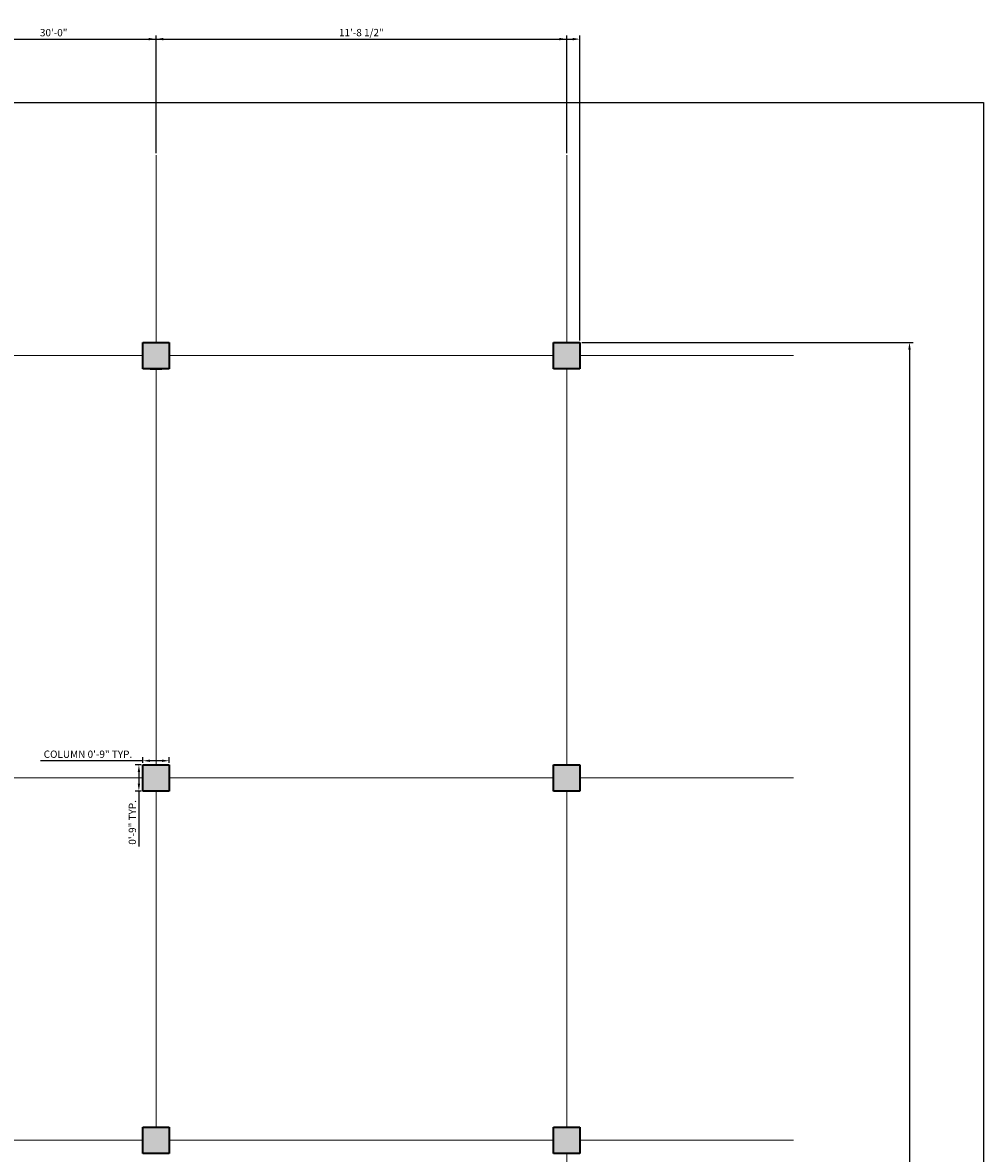
# Model space of a CAD drawing. Units: inches. Extents: x 2169 to 10664, y 1669 to 6352.
# Tile 7 of 17: x 2922 to 3251, y 2479 to 2866. Entities that reach past the tile are written whole.
import ezdxf

# ---------------------------------------------------------------- set-up
doc = ezdxf.new("R2010")
doc.units = ezdxf.units.IN
for name, color, linetype, lineweight in [('A-ANNO-DIMS', 3, 'Continuous', 18), ('A-ANNO-TTLB', 7, 'Continuous', 25), ('A-COLS', 3, 'Continuous', 35), ('A-COLS-PATT', 3, 'Continuous', 13), ('A-GRID', 1, 'Continuous', 13)]:
    doc.layers.add(name, color=color, linetype=linetype, lineweight=lineweight)
doc.styles.get("Standard").update_dxf_attribs({"font": 'arial.ttf'})
doc.dimstyles.new('ISO-25', dxfattribs={"dimtxt": 2.5, "dimasz": 2.5, "dimexe": 1.25, "dimexo": 0.625, "dimtad": 1, "dimdec": 0, "dimlunit": 3, "dimtxsty": 'Standard', "dimcen": 2.5, "dimadec": 0, "dimazin": 0, "dimtfac": 1, "dimtdec": 0, "dimtmove": 0, "dimatfit": 3, "dimfxl": 1, "dimarcsym": 0})

# ---------------------------------------------------------------- blocks, each defined once
blk = doc.blocks.new('COL-9X9')
for p, q in [((0, 9), (9, 9)), ((0, 0), (0, 9)), ((9, 9), (9, 0)), ((9, 0), (0, 0))]:
    blk.add_line(p, q)
blk = doc.blocks.new('*D51')
at = {"layer": 'A-ANNO-DIMS', "color": 0, "lineweight": -2, "transparency": 16777216}
for p, q in [((2963.57, 2613.03), (2928.51, 2613.03)), ((2963.57, 2612.31), (2963.57, 2614.28)), ((2970.07, 2613.03), (2966.07, 2613.03)), ((2972.57, 2612.31), (2972.57, 2614.28))]:
    blk.add_line(p, q, dxfattribs=at)
at = {"layer": 'A-ANNO-DIMS', "color": 0, "transparency": 16777216}
for points in [[(2966.07, 2613.45), (2966.07, 2612.61), (2963.57, 2613.03)], [(2970.07, 2613.45), (2970.07, 2612.61), (2972.57, 2613.03)]]:
    blk.add_solid(points, dxfattribs=at)
at = {"layer": 'Defpoints', "color": 0, "transparency": 16777216}
for p in [(2963.57, 2613.03), (2963.57, 2611.68), (2972.57, 2611.68)]:
    blk.add_point(p, dxfattribs=at)
at = {"layer": 'A-ANNO-DIMS', "color": 0, "transparency": 16777216, "insert": (2944.79, 2614.95), "char_height": 2.5, "attachment_point": 5}
blk.add_mtext('COLUMN 0\'-9" TYP.', dxfattribs=at)
blk = doc.blocks.new('*D52')
at = {"layer": 'A-ANNO-DIMS', "color": 0, "lineweight": -2, "transparency": 16777216}
for p, q in [((2962.95, 2611.68), (2960.97, 2611.68)), ((2962.22, 2609.18), (2962.22, 2605.18)), ((2962.95, 2602.68), (2960.97, 2602.68)), ((2962.22, 2602.68), (2962.22, 2583.69))]:
    blk.add_line(p, q, dxfattribs=at)
at = {"layer": 'A-ANNO-DIMS', "color": 0, "transparency": 16777216}
for points in [[(2961.81, 2609.18), (2962.64, 2609.18), (2962.22, 2611.68)], [(2961.81, 2605.18), (2962.64, 2605.18), (2962.22, 2602.68)]]:
    blk.add_solid(points, dxfattribs=at)
at = {"layer": 'Defpoints', "color": 0, "transparency": 16777216}
for p in [(2963.57, 2611.68), (2962.22, 2602.68), (2963.57, 2602.68)]:
    blk.add_point(p, dxfattribs=at)
at = {"layer": 'A-ANNO-DIMS', "color": 0, "transparency": 16777216, "insert": (2960.32, 2591.94), "char_height": 2.5, "attachment_point": 5, "rotation": 90}
blk.add_mtext('0\'-9" TYP.', dxfattribs=at)
blk = doc.blocks.new('*D85')
at = {"layer": 'A-ANNO-DIMS', "color": 0, "lineweight": -2, "transparency": 16777216}
for p, q in [((2757.57, 2820.9), (2757.57, 2861.22)), ((2760.07, 2859.97), (2965.57, 2859.97)), ((2968.07, 2820.9), (2968.07, 2861.22))]:
    blk.add_line(p, q, dxfattribs=at)
at = {"layer": 'A-ANNO-DIMS', "color": 0, "transparency": 16777216}
for points in [[(2760.07, 2860.39), (2760.07, 2859.55), (2757.57, 2859.97)], [(2965.57, 2860.39), (2965.57, 2859.55), (2968.07, 2859.97)]]:
    blk.add_solid(points, dxfattribs=at)
at = {"layer": 'Defpoints', "color": 0, "transparency": 16777216}
for p in [(2968.07, 2859.97), (2757.57, 2820.27), (2968.07, 2820.27)]:
    blk.add_point(p, dxfattribs=at)
at = {"layer": 'A-ANNO-DIMS', "color": 0, "transparency": 16777216, "insert": (2862.82, 2861.89), "char_height": 2.5, "attachment_point": 5}
blk.add_mtext('17\'-6 1/2"', dxfattribs=at)
blk = doc.blocks.new('*D86')
at = {"layer": 'A-ANNO-DIMS', "color": 0, "lineweight": -2, "transparency": 16777216}
for p, q in [((2968.07, 2820.9), (2968.07, 2861.22)), ((2970.57, 2859.97), (3106.07, 2859.97)), ((3108.57, 2820.9), (3108.57, 2861.22))]:
    blk.add_line(p, q, dxfattribs=at)
at = {"layer": 'A-ANNO-DIMS', "color": 0, "transparency": 16777216}
for points in [[(2970.57, 2860.39), (2970.57, 2859.55), (2968.07, 2859.97)], [(3106.07, 2860.39), (3106.07, 2859.55), (3108.57, 2859.97)]]:
    blk.add_solid(points, dxfattribs=at)
at = {"layer": 'Defpoints', "color": 0, "transparency": 16777216}
for p in [(3108.57, 2859.97), (2968.07, 2820.27), (3108.57, 2820.27)]:
    blk.add_point(p, dxfattribs=at)
at = {"layer": 'A-ANNO-DIMS', "color": 0, "transparency": 16777216, "insert": (3038.32, 2861.89), "char_height": 2.5, "attachment_point": 5}
blk.add_mtext('11\'-8 1/2"', dxfattribs=at)
blk = doc.blocks.new('*D91')
at = {"layer": 'A-ANNO-DIMS', "color": 0, "lineweight": -2, "transparency": 16777216}
for p, q in [((2753.07, 2756.81), (2753.07, 2861.22)), ((2755.57, 2859.97), (3110.57, 2859.97)), ((3113.07, 2756.81), (3113.07, 2861.22))]:
    blk.add_line(p, q, dxfattribs=at)
at = {"layer": 'A-ANNO-DIMS', "color": 0, "transparency": 16777216}
for points in [[(2755.57, 2860.39), (2755.57, 2859.55), (2753.07, 2859.97)], [(3110.57, 2860.39), (3110.57, 2859.55), (3113.07, 2859.97)]]:
    blk.add_solid(points, dxfattribs=at)
at = {"layer": 'Defpoints', "color": 0, "transparency": 16777216}
for p in [(3113.07, 2859.97), (2753.07, 2756.18), (3113.07, 2756.18)]:
    blk.add_point(p, dxfattribs=at)
at = {"layer": 'A-ANNO-DIMS', "color": 0, "transparency": 16777216, "insert": (2933.07, 2861.87), "char_height": 2.5, "attachment_point": 5}
blk.add_mtext('30\'-0"', dxfattribs=at)
blk = doc.blocks.new('*D92')
at = {"layer": 'A-ANNO-DIMS', "color": 0, "lineweight": -2, "transparency": 16777216}
for p, q in [((3113.7, 2756.18), (3227.1, 2756.18)), ((3225.85, 2753.68), (3225.85, 2158.68)), ((3113.7, 2156.18), (3227.1, 2156.18))]:
    blk.add_line(p, q, dxfattribs=at)
at = {"layer": 'A-ANNO-DIMS', "color": 0, "transparency": 16777216}
for points in [[(3225.43, 2753.68), (3226.27, 2753.68), (3225.85, 2756.18)], [(3225.43, 2158.68), (3226.27, 2158.68), (3225.85, 2156.18)]]:
    blk.add_solid(points, dxfattribs=at)
at = {"layer": 'Defpoints', "color": 0, "transparency": 16777216}
for p in [(3113.07, 2756.18), (3113.07, 2156.18), (3225.85, 2156.18)]:
    blk.add_point(p, dxfattribs=at)
at = {"layer": 'A-ANNO-DIMS', "color": 0, "transparency": 16777216, "insert": (3223.95, 2456.18), "char_height": 2.5, "attachment_point": 5, "rotation": 90}
blk.add_mtext('50\'-0"', dxfattribs=at)

msp = doc.modelspace()

# ---------------------------------------------------------------- hatches: boundary and pattern name
at = {"layer": 'A-COLS-PATT'}
h = msp.add_hatch(color=256, dxfattribs=at)
h.dxf.hatch_style = 1
h.paths.add_polyline_path([(2762.07, 2165.18), (2753.07, 2165.18), (2753.07, 2156.18), (2762.07, 2156.18)])
h.paths.add_polyline_path([(2972.57, 2165.18), (2963.57, 2165.18), (2963.57, 2156.18), (2972.57, 2156.18)])
h.paths.add_polyline_path([(3113.07, 2165.18), (3104.07, 2165.18), (3104.07, 2156.18), (3113.07, 2156.18)])
h.paths.add_polyline_path([(3113.07, 2330.18), (3113.07, 2339.18), (3104.07, 2339.18), (3104.07, 2330.18)])
h.paths.add_polyline_path([(2972.57, 2339.18), (2963.57, 2339.18), (2963.57, 2330.18), (2972.57, 2330.18)])
h.paths.add_polyline_path([(2762.07, 2330.18), (2762.07, 2339.18), (2753.07, 2339.18), (2753.07, 2330.18)])
h.paths.add_polyline_path([(2753.07, 2478.68), (2762.07, 2478.68), (2762.07, 2487.68), (2753.07, 2487.68)])
h.paths.add_polyline_path([(2963.57, 2487.68), (2963.57, 2478.68), (2972.57, 2478.68), (2972.57, 2487.68)])
h.paths.add_polyline_path([(3104.07, 2487.68), (3104.07, 2478.68), (3113.07, 2478.68), (3113.07, 2487.68)])
h.paths.add_polyline_path([(3104.07, 2602.68), (3113.07, 2602.68), (3113.07, 2611.68), (3104.07, 2611.68)])
h.paths.add_polyline_path([(2963.57, 2602.68), (2972.57, 2602.68), (2972.57, 2611.68), (2963.57, 2611.68)])
h.paths.add_polyline_path([(2753.07, 2611.68), (2753.07, 2602.68), (2762.07, 2602.68), (2762.07, 2611.68)])
h.paths.add_polyline_path([(2762.07, 2747.18), (2762.07, 2756.18), (2753.07, 2756.18), (2753.07, 2747.18)])
h.paths.add_polyline_path([(2972.57, 2747.18), (2972.57, 2756.18), (2963.57, 2756.18), (2963.57, 2747.18)])
h.paths.add_polyline_path([(3104.07, 2756.18), (3104.07, 2747.18), (3113.07, 2747.18), (3113.07, 2756.18)])

# ---------------------------------------------------------------- linework, layer by layer
at = {"layer": 'A-ANNO-TTLB'}
msp.add_lwpolyline([(2169.45, 2838.28), (3251.13, 2838.28), (3251.13, 1669.34), (2169.45, 1669.34)], close=True, dxfattribs=at)
at = {"layer": 'A-COLS'}
for p, q in [((2966.07, 2747.18), (2970.07, 2747.18)), ((3104.07, 2481.18), (3104.07, 2485.18))]:
    msp.add_line(p, q, dxfattribs=at)
at = {"layer": 'A-GRID'}
for p, q in [((2968.07, 2820.27), (2968.07, 2756.18)), ((3108.57, 2820.27), (3108.57, 2756.18)), ((2762.07, 2751.68), (2963.57, 2751.68)), ((2972.57, 2751.68), (3104.07, 2751.68)), ((3113.07, 2751.68), (3186.15, 2751.68)), ((2968.07, 2747.18), (2968.07, 2611.68)), ((3108.57, 2747.18), (3108.57, 2611.68)), ((2762.07, 2607.18), (2963.57, 2607.18)), ((2972.57, 2607.18), (3104.07, 2607.18)), ((3113.07, 2607.18), (3186.15, 2607.18)), ((2968.07, 2602.68), (2968.07, 2487.68)), ((3108.57, 2602.68), (3108.57, 2487.68)), ((2963.57, 2483.18), (2762.07, 2483.18)), ((3104.07, 2483.18), (2972.57, 2483.18)), ((3186.15, 2483.18), (3113.07, 2483.18)), ((3108.57, 2478.68), (3108.57, 2339.18))]:
    msp.add_line(p, q, dxfattribs=at)

# ---------------------------------------------------------------- block references
at = {"layer": 'A-COLS', "rotation": 180}
for p in [(2972.57, 2756.18), (3113.07, 2756.18), (2972.57, 2611.68), (3113.07, 2611.68), (2972.57, 2487.68), (3113.07, 2487.68)]:
    msp.add_blockref('COL-9X9', p, dxfattribs=at)

# ---------------------------------------------------------------- dimensions: what is measured, and where the dimension line sits
at = {"layer": 'A-ANNO-DIMS'}
for base, p1, p2, picture, middle in [((3113.07, 2859.97), (2753.07, 2756.18), (3113.07, 2756.18), '*D91', (2933.07, 2861.87)), ((2968.07, 2859.97), (2757.57, 2820.27), (2968.07, 2820.27), '*D85', (2862.82, 2861.89)), ((3108.57, 2859.97), (2968.07, 2820.27), (3108.57, 2820.27), '*D86', (3038.32, 2861.89))]:
    dim = msp.add_linear_dim(base=base, p1=p1, p2=p2, dimstyle='ISO-25', override={"dimdec": 1, "dimlfac": 1, "dimrnd": 0, "dimzin": 1, "dimdsep": 46, "dimlunit": 4, "dimfrac": 2}, dxfattribs=at)
    dim.commit()
    dim.dimension.update_dxf_attribs({"geometry": picture, "text_midpoint": middle})
dim = msp.add_linear_dim(base=(3225.85, 2156.18), p1=(3113.07, 2756.18), p2=(3113.07, 2156.18), angle=90, dimstyle='ISO-25', override={"dimdec": 1, "dimlfac": 1, "dimrnd": 0, "dimzin": 1, "dimdsep": 46, "dimlunit": 4, "dimfrac": 2}, dxfattribs=at)
dim.commit()
dim.dimension.update_dxf_attribs({"geometry": '*D92', "text_midpoint": (3223.95, 2456.18)})
for base, p1, p2, angle, text, picture, middle in [((2963.57, 2613.03), (2972.57, 2611.68), (2963.57, 2611.68), 180, 'COLUMN <> TYP.', '*D51', (2944.79, 2614.95)), ((2962.22, 2602.68), (2963.57, 2611.68), (2963.57, 2602.68), 270, '<> TYP.', '*D52', (2960.32, 2591.94))]:
    dim = msp.add_linear_dim(base=base, p1=p1, p2=p2, angle=angle, text=text, dimstyle='ISO-25', override={"dimdec": 1, "dimlfac": 1, "dimrnd": 0, "dimzin": 1, "dimdsep": 46, "dimlunit": 4, "dimfrac": 2}, dxfattribs=at)
    dim.commit()
    dim.dimension.update_dxf_attribs({"geometry": picture, "text_midpoint": middle})

doc.saveas('drawing.dxf')
